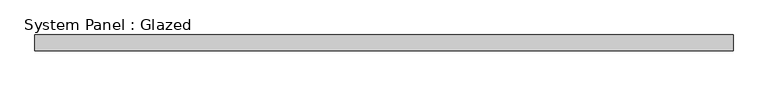
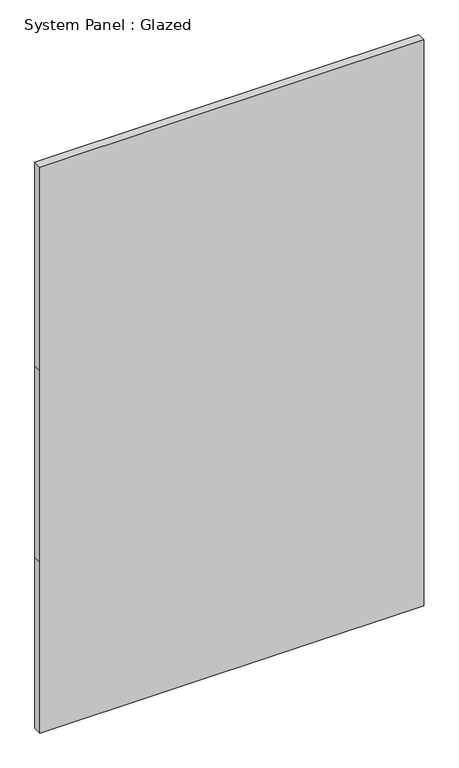
"""IFC4 building model written with IfcOpenShell, lengths in millimetres: plate geometry, System Panel : Glazed."""

from ifc_helpers import new_model, si_unit, frame, origin, place, context, project, spatial, polyline, outline, extrude, source, transform, mapped, element, save


def system_panel_glazed_b2f512c6(model_context):
    return source(origin(), model_context, "Body", "SweptSolid", [
        extrude(outline(polyline([(0.0, -561.975), (0.0, 561.975), (529.155826, 561.975), (1121.8116521, 561.975), (1751.7137588, 561.975), (1751.7137588, -561.975), (1121.8116521, -561.975), (529.155826, -561.975), (0.0, -561.975)])), frame((0.0, 19.05, 0.0), z_axis=(0.0, 1.0, 0.0), x_axis=(0.0, 0.0, 1.0)), (0.0, 0.0, 1.0), 25.4),
    ])


if __name__ == "__main__":
    model = new_model("IFC4")
    model_context = context("Model", 3, world=origin())
    ifc_project = project(units=[si_unit("LENGTHUNIT", "METRE", prefix="MILLI")], contexts=[model_context])
    site = spatial("IfcSite", under=ifc_project)
    building = spatial("IfcBuilding", under=site)
    placement = place(None, origin())
    system_panel_glazed_shape = system_panel_glazed_b2f512c6(model_context)
    element("IfcPlate", 1, ObjectType="System Panel : Glazed", at=placement, inside=building, context=model_context, shape_type="MappedRepresentation", body=[
        mapped(system_panel_glazed_shape, transform((0.0, 0.0, 0.0), x_axis=(1.0, 0.0, 0.0), y_axis=(0.0, 1.0, 0.0), z_axis=(0.0, 0.0, 1.0))),
    ])
    save(model, "model.ifc")

# Revit data of these elements
# Type "System Panel : Glazed"
#   Construction Type Id = "GSP4R"
#   Analytic Construction = "1/8 in Pilkington single glazing"
#   Visual Light Transmittance = 0.9
#   Solar Heat Gain Coefficient = 0.86
#   Heat Transfer Coefficient (U) = 1.18115 BTU/(h·ft²·°F)
#   Define Thermal Properties by = 1
# Element 1 (IfcPlate, "System Panel : Glazed")
#   Materials on its faces: "Glass"
# Materials
#   "Glass": class "Glass", colour RGB 0 128 192, transparency 0.75, Description = "Soda Lime Glass", Cost = 0
